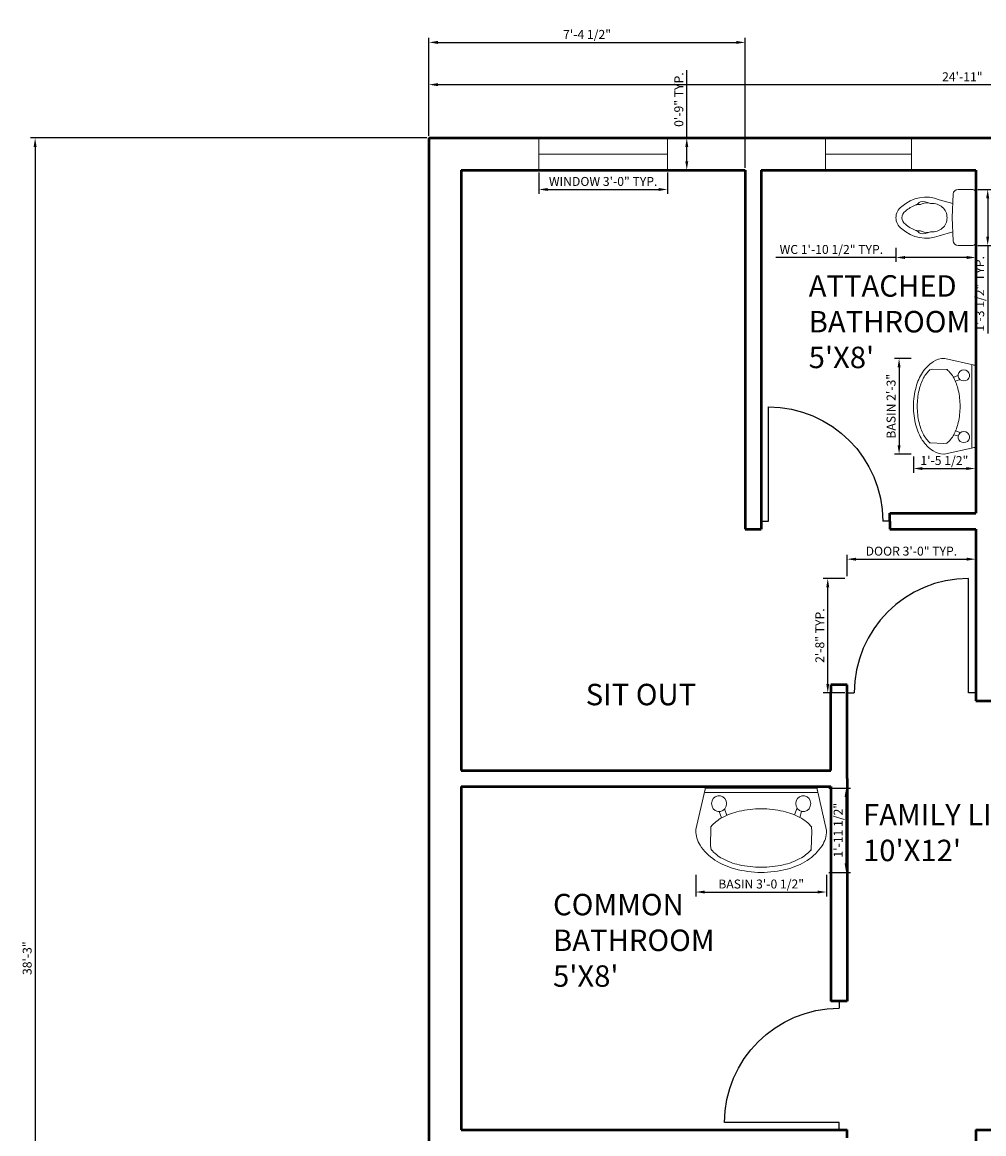
# Model space of a CAD drawing. Units: inches. Extents: x 20697 to 21575, y 6189 to 6822.
# Tile 6 of 7: x 21134 to 21403, y 6511 to 6822. Entities that reach past the tile are written whole.
import ezdxf

# ---------------------------------------------------------------- set-up
doc = ezdxf.new("R2010")
doc.units = ezdxf.units.IN
for name, color, linetype, lineweight in [('A-ANNO-DIMS', 2, 'Continuous', 18), ('A-AREA-IDEN', 7, 'Continuous', 18), ('A-DOOR', 4, 'Continuous', 25), ('A-FLOR-FIXT', 9, 'Continuous', 18), ('A-GLAZ', 4, 'Continuous', 18), ('A-WALL', 7, 'Continuous', 50)]:
    doc.layers.add(name, color=color, linetype=linetype, lineweight=lineweight)
doc.styles.get("Standard").update_dxf_attribs({"font": 'arial.ttf'})
doc.dimstyles.new('ISO-25', dxfattribs={"dimtxt": 2.5, "dimasz": 2.5, "dimexe": 1.25, "dimexo": 0.625, "dimtad": 1, "dimdec": 0, "dimlunit": 3, "dimtxsty": 'Standard', "dimcen": 2.5, "dimadec": 0, "dimazin": 0, "dimtfac": 1, "dimtdec": 0, "dimtmove": 0, "dimatfit": 3, "dimfxl": 1, "dimarcsym": 0})

# ---------------------------------------------------------------- blocks, each defined once
blk = doc.blocks.new('*D1')
at = {"layer": 'A-ANNO-DIMS', "color": 0, "lineweight": -2, "transparency": 16777216}
for p, q in [((21248.16, 6790.38), (21248.16, 6805.94)), ((21546.66, 6790.38), (21546.66, 6805.94)), ((21250.66, 6804.69), (21544.16, 6804.69))]:
    blk.add_line(p, q, dxfattribs=at)
at = {"layer": 'A-ANNO-DIMS', "color": 0, "transparency": 16777216}
for points in [[(21250.66, 6805.11), (21250.66, 6804.27), (21248.16, 6804.69)], [(21544.16, 6805.11), (21544.16, 6804.27), (21546.66, 6804.69)]]:
    blk.add_solid(points, dxfattribs=at)
at = {"layer": 'Defpoints', "color": 0, "transparency": 16777216}
for p in [(21546.66, 6804.69), (21248.16, 6789.76), (21546.66, 6789.76)]:
    blk.add_point(p, dxfattribs=at)
at = {"layer": 'A-ANNO-DIMS', "color": 0, "transparency": 16777216, "insert": (21397.41, 6806.57), "char_height": 2.5, "attachment_point": 5}
blk.add_mtext('24\'-11"', dxfattribs=at)
blk = doc.blocks.new('*D2')
at = {"layer": 'A-ANNO-DIMS', "color": 0, "lineweight": -2, "transparency": 16777216}
for p, q in [((21247.54, 6789.76), (21136.72, 6789.76)), ((21137.97, 6787.26), (21137.97, 6333.26)), ((21247.54, 6330.76), (21136.72, 6330.76))]:
    blk.add_line(p, q, dxfattribs=at)
at = {"layer": 'A-ANNO-DIMS', "color": 0, "transparency": 16777216}
for points in [[(21137.56, 6787.26), (21138.39, 6787.26), (21137.97, 6789.76)], [(21137.56, 6333.26), (21138.39, 6333.26), (21137.97, 6330.76)]]:
    blk.add_solid(points, dxfattribs=at)
at = {"layer": 'Defpoints', "color": 0, "transparency": 16777216}
for p in [(21248.16, 6789.76), (21137.97, 6330.76), (21248.16, 6330.76)]:
    blk.add_point(p, dxfattribs=at)
at = {"layer": 'A-ANNO-DIMS', "color": 0, "transparency": 16777216, "insert": (21136.07, 6560.26), "char_height": 2.5, "attachment_point": 5, "rotation": 90}
blk.add_mtext('38\'-3"', dxfattribs=at)
blk = doc.blocks.new('A$C1308471B')
at = {"ltscale": 20}
for p, q in [((0.0354, 0.4793), (0.1495, 0.4793)), ((0, 0.4607), (0, 0.0186)), ((0.2013, 0.2397), (0.1923, 0.4384)), ((0.1957, 0.3639), (0.3109, 0.3953)), ((0.5021, 0.3528), (0.4724, 0.3528)), ((0.4982, 0.3575), (0.4822, 0.3709)), ((0.2013, 0.2397), (0.1923, 0.0409)), ((0.1959, 0.1193), (0.3109, 0.0879)), ((0.5021, 0.1304), (0.4724, 0.1304)), ((0.4982, 0.1257), (0.4822, 0.1123)), ((0.0354, 0), (0.1495, 0))]:
    blk.add_line(p, q, dxfattribs=at)
for centre, radius, start, end in [((0.0354, 0.4328), 0.0465, 90, 136.52689), ((0.1495, 0.4365), 0.0429, 2.57554, 90), ((0.006, 0.4607), 0.006, 136.52689, 180), ((0.4248, 0.1104), 0.3068, 47.41345, 111.79241), ((0.3654, 0.2416), 0.1206, 83.35226, 180), ((0.3823, 0.3868), 0.0255, 263.35226, 298.57415), ((0.4494, 0.2636), 0.1148, 79.39683, 118.57415), ((0.405, 0.2159), 0.153, 63.50202, 90.45216), ((0.4658, 0.3513), 0.0255, 50, 79.39683), ((0.5146, 0.377), 0.0255, 230, 251.38812), ((0.5021, 0.3273), 0.0255, 70.3751, 90), ((0.4248, 0.1104), 0.2558, 46.61198, 70.3751), ((0.5654, 0.2416), 0.065, 0, 57.29738), ((0.5654, 0.2416), 0.116, 0, 54.71147), ((0.3654, 0.2416), 0.1206, 180, 276.64774), ((0.5654, 0.2416), 0.065, 302.70262, 0), ((0.5654, 0.2416), 0.116, 305.28853, 0), ((0.4248, 0.3728), 0.3068, 248.20759, 312.58655), ((0.3823, 0.0964), 0.0255, 61.42585, 96.64774), ((0.4494, 0.2196), 0.1148, 241.42585, 280.60317), ((0.405, 0.2673), 0.153, 269.54784, 296.49798), ((0.4658, 0.1319), 0.0255, 280.60317, 310), ((0.5146, 0.1062), 0.0255, 108.61188, 130), ((0.5021, 0.1559), 0.0255, 270, 289.6249), ((0.4248, 0.3728), 0.2558, 289.6249, 313.38802), ((0.006, 0.0186), 0.006, 180, 223.47311), ((0.0354, 0.0465), 0.0465, 223.47311, 270), ((0.1495, 0.0429), 0.0429, 270, 357.42446)]:
    blk.add_arc(centre, radius, start, end, dxfattribs=at)
blk = doc.blocks.new('A$C5801748C')
for p, q in [((0.0001, 0.2133), (0.0456, 0.4148)), ((0.0456, 0.42), (0.6044, 0.42)), ((0.0456, 0.4096), (0.0456, 0.42)), ((0.6044, 0.3974), (0.0456, 0.3974)), ((0.6044, 0.42), (0.6044, 0.4096)), ((0.65, 0.2089), (0.6044, 0.4148)), ((0.0803, 0.3556), (0.0781, 0.3423)), ((0.0781, 0.3423), (0.0803, 0.329)), ((0.0868, 0.3673), (0.0803, 0.3556)), ((0.0968, 0.3759), (0.0868, 0.3673)), ((0.109, 0.3806), (0.0968, 0.3759)), ((0.122, 0.3806), (0.109, 0.3806)), ((0.1342, 0.3759), (0.122, 0.3806)), ((0.1441, 0.3673), (0.1342, 0.3759)), ((0.1506, 0.3556), (0.1441, 0.3673)), ((0.1529, 0.3423), (0.1506, 0.3556)), ((0.1506, 0.329), (0.1529, 0.3423)), ((0.4994, 0.3556), (0.4971, 0.3423)), ((0.4971, 0.3423), (0.4994, 0.329)), ((0.5059, 0.3673), (0.4994, 0.3556)), ((0.5158, 0.3759), (0.5059, 0.3673)), ((0.528, 0.3806), (0.5158, 0.3759)), ((0.541, 0.3806), (0.528, 0.3806)), ((0.5532, 0.3759), (0.541, 0.3806)), ((0.5632, 0.3673), (0.5532, 0.3759)), ((0.5697, 0.3556), (0.5632, 0.3673)), ((0.5719, 0.3423), (0.5697, 0.3556)), ((0.5697, 0.329), (0.5719, 0.3423)), ((0.0803, 0.329), (0.0868, 0.3173)), ((0.0868, 0.3173), (0.0968, 0.3086)), ((0.0968, 0.3086), (0.109, 0.304)), ((0.109, 0.304), (0.122, 0.304)), ((0.1161, 0.3037), (0.1274, 0.271)), ((0.122, 0.304), (0.1342, 0.3086)), ((0.1342, 0.3086), (0.1441, 0.3173)), ((0.1428, 0.3162), (0.1546, 0.2838)), ((0.1441, 0.3173), (0.1506, 0.329)), ((0.5045, 0.3208), (0.4912, 0.2859)), ((0.4994, 0.329), (0.5059, 0.3173)), ((0.5059, 0.3173), (0.5158, 0.3086)), ((0.5158, 0.3086), (0.528, 0.304)), ((0.5265, 0.3039), (0.5182, 0.273)), ((0.528, 0.304), (0.541, 0.304)), ((0.541, 0.304), (0.5532, 0.3086)), ((0.5532, 0.3086), (0.5632, 0.3173)), ((0.5632, 0.3173), (0.5697, 0.329)), ((0.0751, 0.2243), (0.0727, 0.1323)), ((0.0752, 0.2281), (0.0751, 0.2277)), ((0.0751, 0.2277), (0.0751, 0.2276)), ((0.0751, 0.2243), (0.0751, 0.2276)), ((0.0754, 0.2284), (0.0752, 0.2281)), ((0.0778, 0.2305), (0.0754, 0.2284)), ((0.578, 0.2053), (0.5751, 0.2235)), ((0.5739, 0.1134), (0.578, 0.2053)), ((0.0727, 0.1323), (0.0761, 0.1135)), ((0.0773, 0.108), (0.0773, 0.108)), ((0.5724, 0.1068), (0.5733, 0.1104))]:
    blk.add_line(p, q)
for centre, radius, start, end in [((0.2883, -0.0209), 0.3337, 102.6999, 117.8694), ((0.3271, -0.213), 0.5296, 90.2298, 102.2344), ((0.3229, -0.213), 0.5296, 77.7656, 89.7702), ((0.3617, -0.0209), 0.3337, 62.1306, 77.3001), ((0.2263, 0.0989), 0.1988, 118.2302, 139.6822), ((0.4237, 0.0989), 0.1989, 39.3299, 61.7657), ((0.1315, 0.2085), 0.1315, 177.9266, 179.8113), ((0.1311, 0.2071), 0.1311, 179.1785, 213.1413), ((0.519, 0.2054), 0.131, 326.4084, 0.3713), ((0.5185, 0.2068), 0.1315, 359.7541, 0.9471), ((0.2279, 0.2678), 0.2454, 212.6461, 237.0936), ((0.2263, 0.2437), 0.1988, 220.8964, 241.7723), ((0.4237, 0.2437), 0.1988, 298.2281, 319.1983), ((0.4226, 0.2669), 0.2453, 302.4413, 326.8887), ((0.29, 0.3671), 0.3625, 237.383, 254.6821), ((0.2883, 0.3635), 0.3337, 242.1306, 257.3001), ((0.3617, 0.3635), 0.3337, 282.6999, 297.8694), ((0.3614, 0.3667), 0.3624, 284.841, 302.14), ((0.3289, 0.527), 0.527, 255.1956, 269.4863), ((0.3271, 0.5556), 0.5296, 257.7656, 269.7702), ((0.3239, 0.527), 0.527, 270.0316, 284.3223), ((0.3229, 0.5556), 0.5296, 270.2298, 282.2344)]:
    blk.add_arc(centre, radius, start, end)
blk = doc.blocks.new('DOOR-SWING-36')
for p, q in [((34, 0), (34, 32)), ((0, 0), (2, 0)), ((36, 0), (34, 0))]:
    blk.add_line(p, q)
blk.add_arc((34, 0), 32, 90, 180)
blk = doc.blocks.new('WIN-36X9')
for p, q in [((0, 9), (36, 9)), ((0, 0), (0, 9)), ((36, 9), (36, 0)), ((0, 4.5), (36, 4.5)), ((36, 0), (0, 0))]:
    blk.add_line(p, q)
blk = doc.blocks.new('WIN-24X9')
for p, q in [((0, 9), (24, 9)), ((0, 0), (0, 9)), ((24, 9), (24, 0)), ((0, 4.5), (24, 4.5)), ((24, 0), (0, 0))]:
    blk.add_line(p, q)
blk = doc.blocks.new('*D20')
at = {"layer": 'A-ANNO-DIMS', "color": 0, "lineweight": -2, "transparency": 16777216}
for p, q in [((21365.16, 6667.13), (21365.16, 6673.16)), ((21367.66, 6671.91), (21398.66, 6671.91)), ((21401.16, 6667.13), (21401.16, 6673.16))]:
    blk.add_line(p, q, dxfattribs=at)
at = {"layer": 'A-ANNO-DIMS', "color": 0, "transparency": 16777216}
for points in [[(21367.66, 6672.32), (21367.66, 6671.49), (21365.16, 6671.91)], [(21398.66, 6672.32), (21398.66, 6671.49), (21401.16, 6671.91)]]:
    blk.add_solid(points, dxfattribs=at)
at = {"layer": 'Defpoints', "color": 0, "transparency": 16777216}
for p in [(21401.16, 6671.91), (21365.16, 6666.51), (21401.16, 6666.51)]:
    blk.add_point(p, dxfattribs=at)
at = {"layer": 'A-ANNO-DIMS', "color": 0, "transparency": 16777216, "insert": (21383.16, 6673.83), "char_height": 2.5, "attachment_point": 5}
blk.add_mtext('DOOR 3\'-0" TYP.', dxfattribs=at)
blk = doc.blocks.new('*D21')
at = {"layer": 'A-ANNO-DIMS', "color": 0, "lineweight": -2, "transparency": 16777216}
for p, q in [((21364.54, 6666.51), (21358.51, 6666.51)), ((21359.76, 6637.01), (21359.76, 6664.01)), ((21364.54, 6634.51), (21358.51, 6634.51))]:
    blk.add_line(p, q, dxfattribs=at)
at = {"layer": 'A-ANNO-DIMS', "color": 0, "transparency": 16777216}
for points in [[(21359.35, 6664.01), (21360.18, 6664.01), (21359.76, 6666.51)], [(21359.35, 6637.01), (21360.18, 6637.01), (21359.76, 6634.51)]]:
    blk.add_solid(points, dxfattribs=at)
at = {"layer": 'Defpoints', "color": 0, "transparency": 16777216}
for p in [(21359.76, 6666.51), (21365.16, 6666.51), (21365.16, 6634.51)]:
    blk.add_point(p, dxfattribs=at)
at = {"layer": 'A-ANNO-DIMS', "color": 0, "transparency": 16777216, "insert": (21357.86, 6650.51), "char_height": 2.5, "attachment_point": 5, "rotation": 90}
blk.add_mtext('2\'-8" TYP.', dxfattribs=at)
blk = doc.blocks.new('*D26')
at = {"layer": 'A-ANNO-DIMS', "color": 0, "lineweight": -2, "transparency": 16777216}
for p, q in [((21278.91, 6780.13), (21278.91, 6774.11)), ((21314.91, 6780.13), (21314.91, 6774.11)), ((21281.41, 6775.36), (21312.41, 6775.36))]:
    blk.add_line(p, q, dxfattribs=at)
at = {"layer": 'A-ANNO-DIMS', "color": 0, "transparency": 16777216}
for points in [[(21281.41, 6775.77), (21281.41, 6774.94), (21278.91, 6775.36)], [(21312.41, 6775.77), (21312.41, 6774.94), (21314.91, 6775.36)]]:
    blk.add_solid(points, dxfattribs=at)
at = {"layer": 'Defpoints', "color": 0, "transparency": 16777216}
for p in [(21278.91, 6780.76), (21314.91, 6780.76), (21314.91, 6775.36)]:
    blk.add_point(p, dxfattribs=at)
at = {"layer": 'A-ANNO-DIMS', "color": 0, "transparency": 16777216, "insert": (21296.91, 6777.28), "char_height": 2.5, "attachment_point": 5}
blk.add_mtext('WINDOW 3\'-0" TYP.', dxfattribs=at)
blk = doc.blocks.new('*D27')
at = {"layer": 'A-ANNO-DIMS', "color": 0, "lineweight": -2, "transparency": 16777216}
for p, q in [((21320.31, 6789.76), (21320.31, 6808.75)), ((21315.54, 6789.76), (21321.56, 6789.76)), ((21320.31, 6783.26), (21320.31, 6787.26)), ((21315.54, 6780.76), (21321.56, 6780.76))]:
    blk.add_line(p, q, dxfattribs=at)
at = {"layer": 'A-ANNO-DIMS', "color": 0, "transparency": 16777216}
for points in [[(21319.9, 6787.26), (21320.73, 6787.26), (21320.31, 6789.76)], [(21319.9, 6783.26), (21320.73, 6783.26), (21320.31, 6780.76)]]:
    blk.add_solid(points, dxfattribs=at)
at = {"layer": 'Defpoints', "color": 0, "transparency": 16777216}
for p in [(21314.91, 6789.76), (21320.31, 6789.76), (21314.91, 6780.76)]:
    blk.add_point(p, dxfattribs=at)
at = {"layer": 'A-ANNO-DIMS', "color": 0, "transparency": 16777216, "insert": (21318.41, 6800.5), "char_height": 2.5, "attachment_point": 5, "rotation": 90}
blk.add_mtext('0\'-9" TYP.', dxfattribs=at)
blk = doc.blocks.new('*D34')
at = {"layer": 'A-ANNO-DIMS', "color": 0, "lineweight": -2, "transparency": 16777216}
for p, q in [((21378.84, 6759.05), (21378.84, 6755.08)), ((21401.16, 6759.05), (21401.16, 6755.08)), ((21378.84, 6756.33), (21345.19, 6756.33)), ((21398.66, 6756.33), (21381.34, 6756.33))]:
    blk.add_line(p, q, dxfattribs=at)
at = {"layer": 'A-ANNO-DIMS', "color": 0, "transparency": 16777216}
for points in [[(21381.34, 6756.74), (21381.34, 6755.91), (21378.84, 6756.33)], [(21398.66, 6756.74), (21398.66, 6755.91), (21401.16, 6756.33)]]:
    blk.add_solid(points, dxfattribs=at)
at = {"layer": 'Defpoints', "color": 0, "transparency": 16777216}
for p in [(21378.84, 6759.68), (21401.16, 6759.68), (21378.84, 6756.33)]:
    blk.add_point(p, dxfattribs=at)
at = {"layer": 'A-ANNO-DIMS', "color": 0, "transparency": 16777216, "insert": (21360.77, 6758.25), "char_height": 2.5, "attachment_point": 5}
blk.add_mtext('WC 1\'-10 1/2" TYP.', dxfattribs=at)
blk = doc.blocks.new('*D35')
at = {"layer": 'A-ANNO-DIMS', "color": 0, "lineweight": -2, "transparency": 16777216}
for p, q in [((21401.79, 6775.38), (21405.76, 6775.38)), ((21404.51, 6772.88), (21404.51, 6762.18)), ((21401.79, 6759.68), (21405.76, 6759.68)), ((21404.51, 6759.68), (21404.51, 6735.1))]:
    blk.add_line(p, q, dxfattribs=at)
at = {"layer": 'A-ANNO-DIMS', "color": 0, "transparency": 16777216}
for points in [[(21404.09, 6772.88), (21404.93, 6772.88), (21404.51, 6775.38)], [(21404.09, 6762.18), (21404.93, 6762.18), (21404.51, 6759.68)]]:
    blk.add_solid(points, dxfattribs=at)
at = {"layer": 'Defpoints', "color": 0, "transparency": 16777216}
for p in [(21401.16, 6775.38), (21401.16, 6759.68), (21404.51, 6759.68)]:
    blk.add_point(p, dxfattribs=at)
at = {"layer": 'A-ANNO-DIMS', "color": 0, "transparency": 16777216, "insert": (21402.59, 6746.14), "char_height": 2.5, "attachment_point": 5, "rotation": 90}
blk.add_mtext('1\'-3 1/2" TYP.', dxfattribs=at)
blk = doc.blocks.new('*D36')
at = {"layer": 'A-ANNO-DIMS', "color": 0, "lineweight": -2, "transparency": 16777216}
for p, q in [((21383.11, 6728.09), (21378.47, 6728.09)), ((21379.72, 6725.59), (21379.72, 6703.8)), ((21383.11, 6701.3), (21378.47, 6701.3))]:
    blk.add_line(p, q, dxfattribs=at)
at = {"layer": 'A-ANNO-DIMS', "color": 0, "transparency": 16777216}
for points in [[(21379.3, 6725.59), (21380.13, 6725.59), (21379.72, 6728.09)], [(21379.3, 6703.8), (21380.13, 6703.8), (21379.72, 6701.3)]]:
    blk.add_solid(points, dxfattribs=at)
at = {"layer": 'Defpoints', "color": 0, "transparency": 16777216}
for p in [(21383.74, 6728.09), (21379.72, 6701.3), (21383.74, 6701.3)]:
    blk.add_point(p, dxfattribs=at)
at = {"layer": 'A-ANNO-DIMS', "color": 0, "transparency": 16777216, "insert": (21377.8, 6714.69), "char_height": 2.5, "attachment_point": 5, "rotation": 90}
blk.add_mtext('BASIN 2\'-3"', dxfattribs=at)
blk = doc.blocks.new('*D37')
at = {"layer": 'A-ANNO-DIMS', "color": 0, "lineweight": -2, "transparency": 16777216}
for p, q in [((21383.74, 6700.67), (21383.74, 6696.03)), ((21401.03, 6700.67), (21401.03, 6696.03)), ((21386.24, 6697.28), (21398.53, 6697.28))]:
    blk.add_line(p, q, dxfattribs=at)
at = {"layer": 'A-ANNO-DIMS', "color": 0, "transparency": 16777216}
for points in [[(21386.24, 6697.69), (21386.24, 6696.86), (21383.74, 6697.28)], [(21398.53, 6697.69), (21398.53, 6696.86), (21401.03, 6697.28)]]:
    blk.add_solid(points, dxfattribs=at)
at = {"layer": 'Defpoints', "color": 0, "transparency": 16777216}
for p in [(21383.74, 6701.3), (21401.03, 6701.3), (21401.03, 6697.28)]:
    blk.add_point(p, dxfattribs=at)
at = {"layer": 'A-ANNO-DIMS', "color": 0, "transparency": 16777216, "insert": (21392.39, 6699.19), "char_height": 2.5, "attachment_point": 5}
blk.add_mtext('1\'-5 1/2"', dxfattribs=at)
blk = doc.blocks.new('*D38')
at = {"layer": 'A-ANNO-DIMS', "color": 0, "lineweight": -2, "transparency": 16777216}
for p, q in [((21322.84, 6583.63), (21322.84, 6577.52)), ((21359.41, 6583.63), (21359.41, 6577.52)), ((21325.34, 6578.77), (21356.91, 6578.77))]:
    blk.add_line(p, q, dxfattribs=at)
at = {"layer": 'A-ANNO-DIMS', "color": 0, "transparency": 16777216}
for points in [[(21325.34, 6579.19), (21325.34, 6578.35), (21322.84, 6578.77)], [(21356.91, 6579.19), (21356.91, 6578.35), (21359.41, 6578.77)]]:
    blk.add_solid(points, dxfattribs=at)
at = {"layer": 'Defpoints', "color": 0, "transparency": 16777216}
for p in [(21322.84, 6584.26), (21359.41, 6584.26), (21359.41, 6578.77)]:
    blk.add_point(p, dxfattribs=at)
at = {"layer": 'A-ANNO-DIMS', "color": 0, "transparency": 16777216, "insert": (21341.13, 6580.69), "char_height": 2.5, "attachment_point": 5}
blk.add_mtext('BASIN 3\'-0 1/2"', dxfattribs=at)
blk = doc.blocks.new('*D39')
at = {"layer": 'A-ANNO-DIMS', "color": 0, "lineweight": -2, "transparency": 16777216}
for p, q in [((21360.04, 6607.86), (21366.15, 6607.86)), ((21364.9, 6586.76), (21364.9, 6605.36)), ((21360.04, 6584.26), (21366.15, 6584.26))]:
    blk.add_line(p, q, dxfattribs=at)
at = {"layer": 'A-ANNO-DIMS', "color": 0, "transparency": 16777216}
for points in [[(21364.48, 6605.36), (21365.31, 6605.36), (21364.9, 6607.86)], [(21364.48, 6586.76), (21365.31, 6586.76), (21364.9, 6584.26)]]:
    blk.add_solid(points, dxfattribs=at)
at = {"layer": 'Defpoints', "color": 0, "transparency": 16777216}
for p in [(21359.41, 6607.86), (21364.9, 6607.86), (21359.41, 6584.26)]:
    blk.add_point(p, dxfattribs=at)
at = {"layer": 'A-ANNO-DIMS', "color": 0, "transparency": 16777216, "insert": (21362.98, 6596.06), "char_height": 2.5, "attachment_point": 5, "rotation": 90}
blk.add_mtext('1\'-11 1/2"', dxfattribs=at)
blk = doc.blocks.new('*D68')
at = {"layer": 'A-ANNO-DIMS', "color": 0, "lineweight": -2, "transparency": 16777216}
for p, q in [((21248.16, 6790.38), (21248.16, 6817.76)), ((21336.66, 6781.38), (21336.66, 6817.76)), ((21250.66, 6816.51), (21334.16, 6816.51))]:
    blk.add_line(p, q, dxfattribs=at)
at = {"layer": 'A-ANNO-DIMS', "color": 0, "transparency": 16777216}
for points in [[(21250.66, 6816.92), (21250.66, 6816.09), (21248.16, 6816.51)], [(21334.16, 6816.92), (21334.16, 6816.09), (21336.66, 6816.51)]]:
    blk.add_solid(points, dxfattribs=at)
at = {"layer": 'Defpoints', "color": 0, "transparency": 16777216}
for p in [(21336.66, 6816.51), (21248.16, 6789.76), (21336.66, 6780.76)]:
    blk.add_point(p, dxfattribs=at)
at = {"layer": 'A-ANNO-DIMS', "color": 0, "transparency": 16777216, "insert": (21292.41, 6818.42), "char_height": 2.5, "attachment_point": 5}
blk.add_mtext('7\'-4 1/2"', dxfattribs=at)

msp = doc.modelspace()

# ---------------------------------------------------------------- linework, layer by layer
at = {"layer": 'A-WALL'}
for p, q in [((21248.16, 6789.76), (21248.16, 6330.76)), ((21248.16, 6789.76), (21546.66, 6789.76)), ((21257.16, 6780.76), (21336.66, 6780.76)), ((21257.16, 6780.76), (21257.16, 6612.76)), ((21336.66, 6780.76), (21336.66, 6680.26)), ((21341.16, 6780.76), (21341.16, 6680.26)), ((21341.16, 6780.76), (21401.16, 6780.76)), ((21401.16, 6780.76), (21401.16, 6684.76)), ((21341.16, 6684.76), (21341.16, 6680.26)), ((21377.16, 6684.76), (21401.16, 6684.76)), ((21377.16, 6682.51), (21377.16, 6684.76)), ((21377.16, 6682.51), (21377.16, 6680.26)), ((21336.66, 6680.26), (21341.16, 6680.26)), ((21377.16, 6680.26), (21401.16, 6680.26)), ((21401.16, 6680.26), (21401.16, 6632.26)), ((21360.66, 6636.76), (21360.66, 6634.51)), ((21365.16, 6636.76), (21360.66, 6636.76)), ((21360.66, 6612.76), (21360.66, 6634.51)), ((21365.16, 6610.51), (21365.16, 6636.76)), ((21401.16, 6636.76), (21401.16, 6632.26)), ((21401.16, 6632.26), (21405.66, 6632.26)), ((21257.16, 6612.76), (21360.66, 6612.76)), ((21365.16, 6610.51), (21365.16, 6608.26)), ((21257.16, 6608.26), (21360.66, 6608.26)), ((21257.16, 6608.26), (21257.16, 6512.26)), ((21360.66, 6608.26), (21360.66, 6548.26)), ((21365.16, 6608.26), (21365.16, 6548.26)), ((21365.16, 6548.26), (21360.66, 6548.26)), ((21257.16, 6512.26), (21365.16, 6512.26)), ((21365.16, 6510.01), (21365.16, 6512.26)), ((21401.16, 6512.26), (21401.16, 6339.76)), ((21401.16, 6512.26), (21537.66, 6512.26))]:
    msp.add_line(p, q, dxfattribs=at)

# ---------------------------------------------------------------- block references
at = {"layer": 'A-DOOR', "extrusion": (0, 0, -1), "zscale": -1}
msp.add_blockref('DOOR-SWING-36', (-21377.16, 6682.51), dxfattribs=at)
at = {"layer": 'A-DOOR'}
msp.add_blockref('DOOR-SWING-36', (21365.16, 6634.51), dxfattribs=at)
at = {"layer": 'A-DOOR', "extrusion": (0, 0, -1), "zscale": -1, "rotation": 269.9999999999998}
msp.add_blockref('DOOR-SWING-36', (-21362.91, 6548.26), dxfattribs=at)
at = {"layer": 'A-FLOR-FIXT'}
for name, p, xscale, yscale, zscale, rotation in [('A$C1308471B', (21401.16, 6775.38), 32.76079773388695, 32.76079773388695, 32.76079773388695, 180), ('A$C5801748C', (21383.74, 6728.07), 41.18418410369762, 41.18418410369762, 41.18418410369762, 270)]:
    msp.add_blockref(name, p, dxfattribs=dict(at, xscale=xscale, yscale=yscale, zscale=zscale, rotation=rotation))
at = {"layer": 'A-FLOR-FIXT', "xscale": 56.21062765499749, "yscale": 56.21062765499749, "zscale": 56.21062765499749}
msp.add_blockref('A$C5801748C', (21322.86, 6584.26), dxfattribs=at)
at = {"layer": 'A-GLAZ'}
for name, p in [('WIN-36X9', (21278.91, 6780.76)), ('WIN-24X9', (21359.16, 6780.76))]:
    msp.add_blockref(name, p, dxfattribs=at)

# ---------------------------------------------------------------- texts
at = {"layer": 'A-AREA-IDEN', "char_height": 6, "attachment_point": 1}
for s, insert in [("ATTACHED\\PBATHROOM\\P5'X8'", (21354.42, 6751.36)), ('SIT OUT', (21292.04, 6637.03)), ("FAMILY LIVING\\P10'X12'", (21369.63, 6603.41)), ("COMMON \\PBATHROOM\\P5'X8'", (21282.89, 6578.26))]:
    msp.add_mtext(s, dxfattribs=dict(at, insert=insert))

# ---------------------------------------------------------------- dimensions: what is measured, and where the dimension line sits
at = {"layer": 'A-ANNO-DIMS'}
for base, p1, p2, override, picture, middle in [((21336.66, 6816.51), (21248.16, 6789.76), (21336.66, 6780.76), {"dimdec": 1, "dimlfac": 1, "dimrnd": 0, "dimzin": 1, "dimdsep": 46, "dimlunit": 4, "dimfrac": 2}, '*D68', (21292.41, 6818.42)), ((21546.66169726, 6804.69035485), (21248.16169726, 6789.75667437), (21546.66169726, 6789.75667437), {"dimclrd": 0, "dimclre": 0, "dimclrt": 0}, '*D1', (21397.41169726, 6806.57047082)), ((21401.03, 6697.28), (21383.74, 6701.3), (21401.03, 6701.3), {"dimdec": 1, "dimlfac": 1, "dimrnd": 0, "dimzin": 1, "dimdsep": 46, "dimlunit": 4, "dimfrac": 2}, '*D37', (21392.39, 6699.19))]:
    dim = msp.add_linear_dim(base=base, p1=p1, p2=p2, dimstyle='ISO-25', override=override, dxfattribs=at)
    dim.commit()
    dim.dimension.update_dxf_attribs({"geometry": picture, "text_midpoint": middle})
for base, p1, p2, angle, text, picture, middle in [((21320.31, 6789.76), (21314.91, 6780.76), (21314.91, 6789.76), 90, '<> TYP.', '*D27', (21318.41, 6800.5)), ((21404.51, 6759.68), (21401.16, 6775.38), (21401.16, 6759.68), 270, '<> TYP.', '*D35', (21402.59, 6746.14)), ((21378.84, 6756.33), (21401.16, 6759.68), (21378.84, 6759.68), 180, 'WC <> TYP.', '*D34', (21360.77, 6758.25)), ((21379.72, 6701.3), (21383.74, 6728.09), (21383.74, 6701.3), 270, 'BASIN <>', '*D36', (21377.8, 6714.69)), ((21359.76, 6666.51), (21365.16, 6634.51), (21365.16, 6666.51), 90, '<> TYP.', '*D21', (21357.86, 6650.51))]:
    dim = msp.add_linear_dim(base=base, p1=p1, p2=p2, angle=angle, text=text, dimstyle='ISO-25', override={"dimdec": 1, "dimlfac": 1, "dimrnd": 0, "dimzin": 1, "dimdsep": 46, "dimlunit": 4, "dimfrac": 2}, dxfattribs=at)
    dim.commit()
    dim.dimension.update_dxf_attribs({"geometry": picture, "text_midpoint": middle})
for base, p1, p2, override, picture, middle in [((21137.97, 6330.76), (21248.16, 6789.76), (21248.16, 6330.76), {"dimclrd": 0, "dimclre": 0, "dimclrt": 0}, '*D2', (21136.07, 6560.26)), ((21364.9, 6607.86), (21359.41, 6584.26), (21359.41, 6607.86), {"dimdec": 1, "dimlfac": 1, "dimrnd": 0, "dimzin": 1, "dimdsep": 46, "dimlunit": 4, "dimfrac": 2}, '*D39', (21362.98, 6596.06))]:
    dim = msp.add_linear_dim(base=base, p1=p1, p2=p2, angle=90, dimstyle='ISO-25', override=override, dxfattribs=at)
    dim.commit()
    dim.dimension.update_dxf_attribs({"geometry": picture, "text_midpoint": middle})
for base, p1, p2, text, picture, middle in [((21314.91, 6775.36), (21278.91, 6780.76), (21314.91, 6780.76), 'WINDOW <> TYP.', '*D26', (21296.91, 6777.28)), ((21401.16, 6671.91), (21365.16, 6666.51), (21401.16, 6666.51), 'DOOR <> TYP.', '*D20', (21383.16, 6673.83)), ((21359.41, 6578.77), (21322.84, 6584.26), (21359.41, 6584.26), 'BASIN <>', '*D38', (21341.13, 6580.69))]:
    dim = msp.add_linear_dim(base=base, p1=p1, p2=p2, text=text, dimstyle='ISO-25', override={"dimdec": 1, "dimlfac": 1, "dimrnd": 0, "dimzin": 1, "dimdsep": 46, "dimlunit": 4, "dimfrac": 2}, dxfattribs=at)
    dim.commit()
    dim.dimension.update_dxf_attribs({"geometry": picture, "text_midpoint": middle})

doc.saveas('drawing.dxf')
